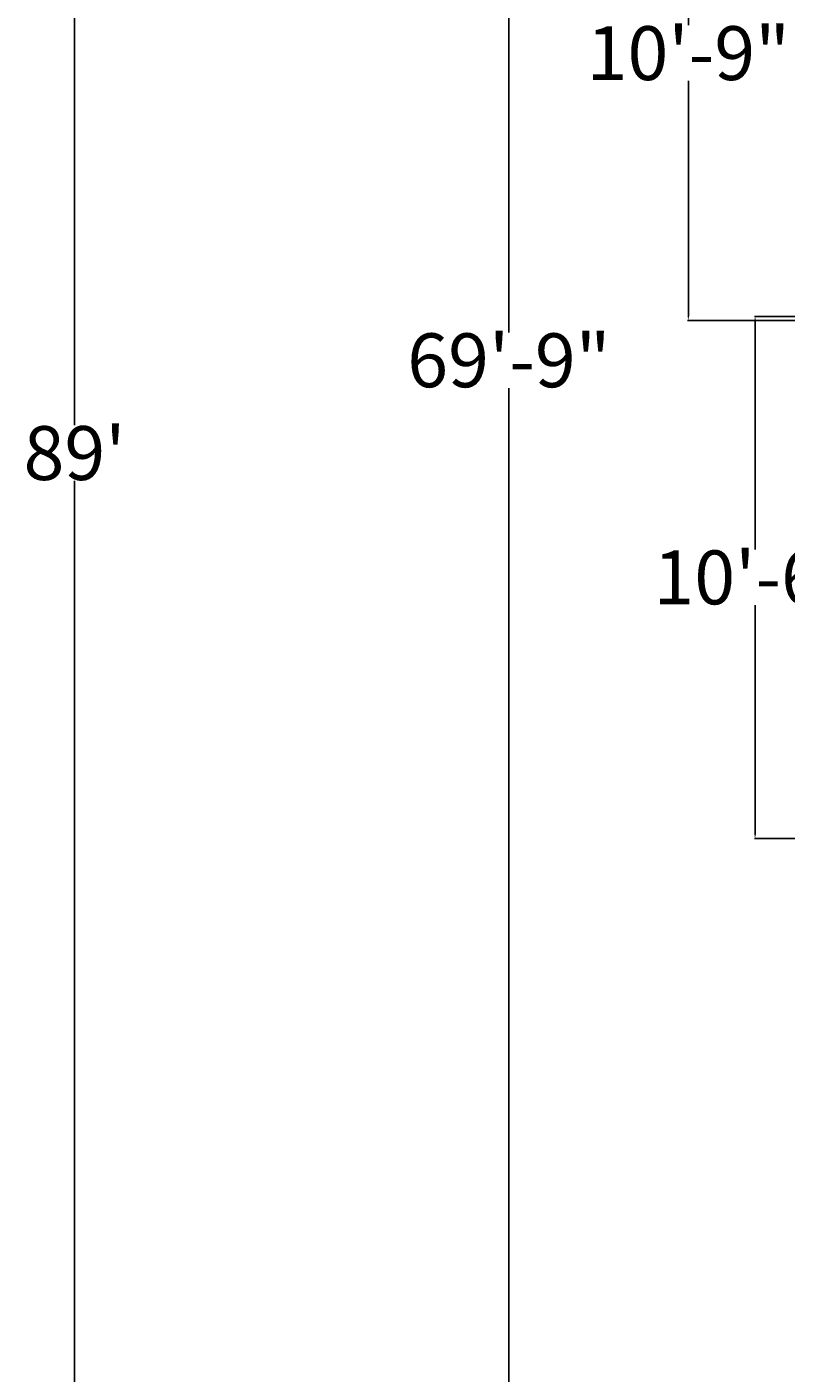
# Model space of a CAD drawing. Units: inches. Extents: x -364 to 705, y -52 to 1250.
# Tile 4 of 34: x -364 to -181, y 323 to 648. Entities that reach past the tile are written whole.
import ezdxf

# ---------------------------------------------------------------- set-up
doc = ezdxf.new("R2010")
doc.units = ezdxf.units.IN
doc.header["$MEASUREMENT"] = 0
doc.layers.add('A-ANNO-DIMS', color=4, linetype='Continuous', lineweight=18)
doc.styles.get("Standard").update_dxf_attribs({"font": 'arial.ttf'})
doc.dimstyles.get("Standard").update_dxf_attribs({"dimtxt": 1, "dimasz": 1, "dimexe": 0.18, "dimexo": 0.0625, "dimgap": 0.09, "dimtad": 0, "dimtih": 1, "dimtoh": 1, "dimdec": 0, "dimzin": 0, "dimdsep": 46, "dimlunit": 3, "dimtxsty": 'Standard', "dimcen": 0.09, "dimadec": 0, "dimazin": 0, "dimtfac": 1, "dimtdec": 0, "dimtofl": 0, "dimtmove": 0, "dimatfit": 3, "dimfxl": 1, "dimtolj": 1, "dimtzin": 0, "dimarcsym": 0})

# ---------------------------------------------------------------- blocks, each defined once
blk = doc.blocks.new('*D18')
at = {"layer": 'A-ANNO-DIMS', "color": 0, "lineweight": -2, "transparency": 16777216}
for p, q in [((-254.46, 1079.11), (-353.05, 1079.11)), ((-352.87, 1078.11), (-352.87, 551.84)), ((-352.87, 12.11), (-352.87, 538.39)), ((-254.46, 11.11), (-353.05, 11.11))]:
    blk.add_line(p, q, dxfattribs=at)
at = {"layer": 'A-ANNO-DIMS', "color": 0, "transparency": 16777216}
for points in [[(-353.04, 1078.11), (-352.7, 1078.11), (-352.87, 1079.11)], [(-353.04, 12.11), (-352.7, 12.11), (-352.87, 11.11)]]:
    blk.add_solid(points, dxfattribs=at)
at = {"layer": 'Defpoints', "color": 0, "transparency": 16777216}
for p in [(-254.4, 1079.11), (-352.87, 11.11), (-254.4, 11.11)]:
    blk.add_point(p, dxfattribs=at)
at = {"layer": 'A-ANNO-DIMS', "color": 0, "transparency": 16777216, "insert": (-352.87, 545.11), "char_height": 1, "width": 1.6985, "attachment_point": 5}
blk.add_mtext("\\A1;{\\H13x;89'}", dxfattribs=at)
blk = doc.blocks.new('*D19')
at = {"layer": 'A-ANNO-DIMS', "color": 0, "lineweight": -2, "transparency": 16777216}
for p, q in [((28.52, 986.11), (-248.33, 986.11)), ((-248.15, 985.11), (-248.15, 574.22)), ((-248.15, 149.87), (-248.15, 560.77)), ((28.52, 148.87), (-248.33, 148.87))]:
    blk.add_line(p, q, dxfattribs=at)
at = {"layer": 'A-ANNO-DIMS', "color": 0, "transparency": 16777216}
for points in [[(-248.32, 985.11), (-247.99, 985.11), (-248.15, 986.11)], [(-248.32, 149.87), (-247.99, 149.87), (-248.15, 148.87)]]:
    blk.add_solid(points, dxfattribs=at)
at = {"layer": 'Defpoints', "color": 0, "transparency": 16777216}
for p in [(28.58, 986.11), (-248.15, 148.87), (28.58, 148.87)]:
    blk.add_point(p, dxfattribs=at)
at = {"layer": 'A-ANNO-DIMS', "color": 0, "transparency": 16777216, "insert": (-248.15, 567.49), "char_height": 1, "attachment_point": 5}
blk.add_mtext('\\A1;{\\H13x;69\'-9"}', dxfattribs=at)
blk = doc.blocks.new('*D30')
at = {"layer": 'A-ANNO-DIMS', "color": 0, "lineweight": -2, "transparency": 16777216}
for p, q in [((28.52, 578.1), (-188.97, 578.1)), ((-188.79, 577.1), (-188.79, 521.83)), ((-188.79, 453.11), (-188.79, 508.38)), ((28.52, 452.11), (-188.97, 452.11))]:
    blk.add_line(p, q, dxfattribs=at)
at = {"layer": 'A-ANNO-DIMS', "color": 0, "transparency": 16777216}
for points in [[(-188.96, 577.1), (-188.63, 577.1), (-188.79, 578.1)], [(-188.96, 453.11), (-188.63, 453.11), (-188.79, 452.11)]]:
    blk.add_solid(points, dxfattribs=at)
at = {"layer": 'Defpoints', "color": 0, "transparency": 16777216}
for p in [(-188.79, 578.1), (28.58, 578.1), (28.58, 452.11)]:
    blk.add_point(p, dxfattribs=at)
at = {"layer": 'A-ANNO-DIMS', "color": 0, "transparency": 16777216, "insert": (-188.79, 515.11), "char_height": 1, "attachment_point": 5}
blk.add_mtext('\\A1;{\\H13x;10\'-6"}', dxfattribs=at)
blk = doc.blocks.new('*D31')
at = {"layer": 'A-ANNO-DIMS', "color": 0, "lineweight": -2, "transparency": 16777216}
for p, q in [((37.52, 706.11), (-205.07, 706.11)), ((-204.89, 705.11), (-204.89, 648.34)), ((-204.89, 578.11), (-204.89, 634.89)), ((37.52, 577.11), (-205.07, 577.11))]:
    blk.add_line(p, q, dxfattribs=at)
at = {"layer": 'A-ANNO-DIMS', "color": 0, "transparency": 16777216}
for points in [[(-205.06, 705.11), (-204.73, 705.11), (-204.89, 706.11)], [(-205.06, 578.11), (-204.73, 578.11), (-204.89, 577.11)]]:
    blk.add_solid(points, dxfattribs=at)
at = {"layer": 'Defpoints', "color": 0, "transparency": 16777216}
for p in [(37.58, 706.11), (-204.89, 577.11), (37.58, 577.11)]:
    blk.add_point(p, dxfattribs=at)
at = {"layer": 'A-ANNO-DIMS', "color": 0, "transparency": 16777216, "insert": (-204.89, 641.61), "char_height": 1, "attachment_point": 5}
blk.add_mtext('\\A1;{\\H13x;10\'-9"}', dxfattribs=at)

msp = doc.modelspace()

# ---------------------------------------------------------------- dimensions: what is measured, and where the dimension line sits
at = {"layer": 'A-ANNO-DIMS'}
for base, p1, p2, picture, middle in [((-352.87, 11.11), (-254.4, 1079.11), (-254.4, 11.11), '*D18', (-352.87, 545.11)), ((-248.15, 148.87), (28.58, 986.11), (28.58, 148.87), '*D19', (-248.15, 567.49)), ((-204.89, 577.11), (37.58, 706.11), (37.58, 577.11), '*D31', (-204.89, 641.61)), ((-188.79, 578.1), (28.58, 452.11), (28.58, 578.1), '*D30', (-188.79, 515.11))]:
    dim = msp.add_linear_dim(base=base, p1=p1, p2=p2, angle=90, text='{\\H13x;<>}', dimstyle='Standard', override={"dimclrd": 0, "dimclre": 0, "dimclrt": 0}, dxfattribs=at)
    dim.commit()
    dim.dimension.update_dxf_attribs({"geometry": picture, "text_midpoint": middle})

doc.saveas('drawing.dxf')
